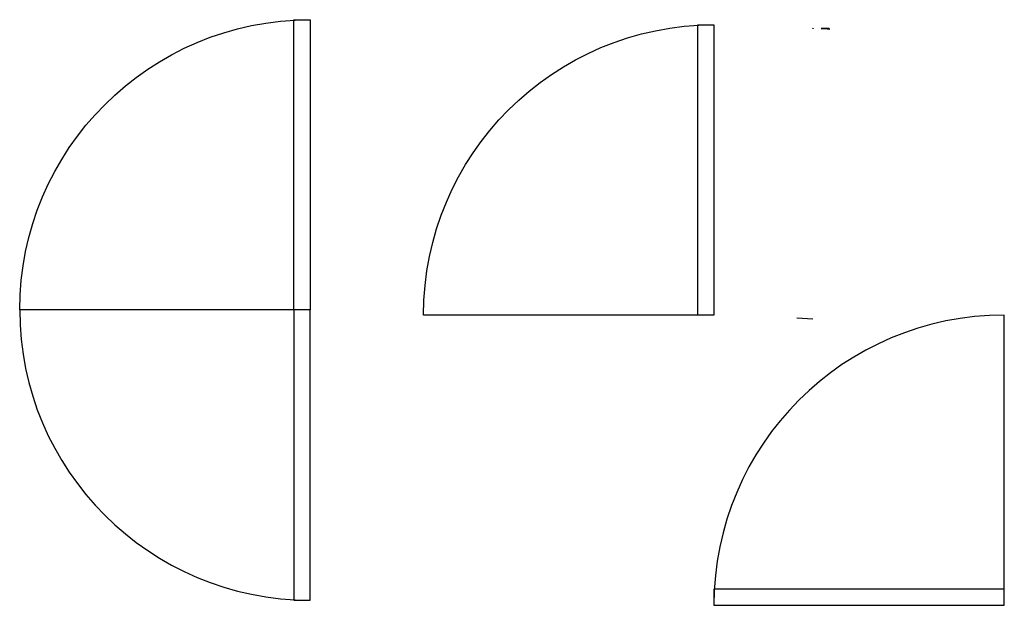
# Model space of a CAD drawing. Units: inches. Extents: x -108 to 1456, y -102 to 617.
# Tile 1 of 8: x -108 to 14, y 414 to 486. Entities that reach past the tile are written whole.
import ezdxf

# ---------------------------------------------------------------- set-up
doc = ezdxf.new("R2010")
doc.units = ezdxf.units.IN
doc.layers.add('A-DOOR', color=3, linetype='Continuous', lineweight=25)

# ---------------------------------------------------------------- blocks, each defined once
blk = doc.blocks.new('DOOR-36-SWING-WITH-CLOSURE')
for p, q in [((36, 36), (0, 36)), ((36, 36), (34, 36)), ((34, 36), (34, 0)), ((36, 0), (36, 36)), ((34, 0), (36, 0))]:
    blk.add_line(p, q)
blk.add_arc((36, 36), 36, 180, 270)

msp = doc.modelspace()

# ---------------------------------------------------------------- linework, layer by layer
at = {"layer": 'A-DOOR'}
for p, q in [((-9.6172, 485.2031), (-9.6234, 485.0917)), ((-9.6188, 485.092), (-9.6188, 485.1476)), ((-7.6203, 485.0921), (-8.6188, 485.1476)), ((-8.6188, 485.1476), (-7.6188, 485.1476)), ((-7.6234, 485.0365), (-7.6203, 485.0921)), ((-7.6188, 485.1476), (-7.6188, 485.036)), ((-11.6157, 449.2586), (-9.6188, 449.1476)), ((-11.6157, 449.2586), (-9.6188, 449.1476))]:
    msp.add_line(p, q, dxfattribs=at)
for centre, start, end in [((-7.6188, 449.1476), 93.184739, 93.192151), ((-7.6188, 449.1476), 90, 91.592369), ((-11.6157, 449.2586), 83.625569, 85.22535)]:
    msp.add_arc(centre, 36, start, end, dxfattribs=at)

# ---------------------------------------------------------------- block references
at = {"layer": 'A-DOOR', "extrusion": (0, 0, -1), "zscale": -1, "rotation": 180}
for p in [(107.97, 486.2363), (57.9006, 485.5981)]:
    msp.add_blockref('DOOR-36-SWING-WITH-CLOSURE', p, dxfattribs=at)
at = {"layer": 'A-DOOR'}
msp.add_blockref('DOOR-36-SWING-WITH-CLOSURE', (-107.97, 414.236), dxfattribs=at)
at = {"layer": 'A-DOOR', "rotation": 269.9999999999998}
msp.add_blockref('DOOR-36-SWING-WITH-CLOSURE', (-21.9005, 449.5981), dxfattribs=at)

doc.saveas('drawing.dxf')
